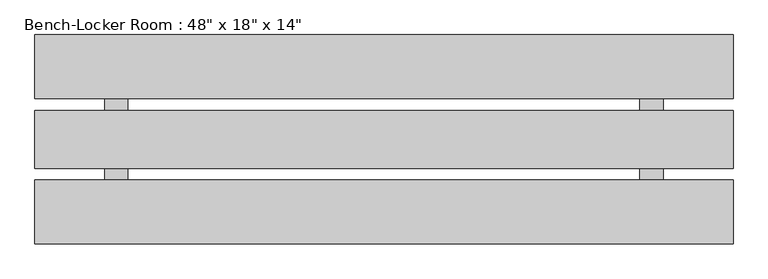
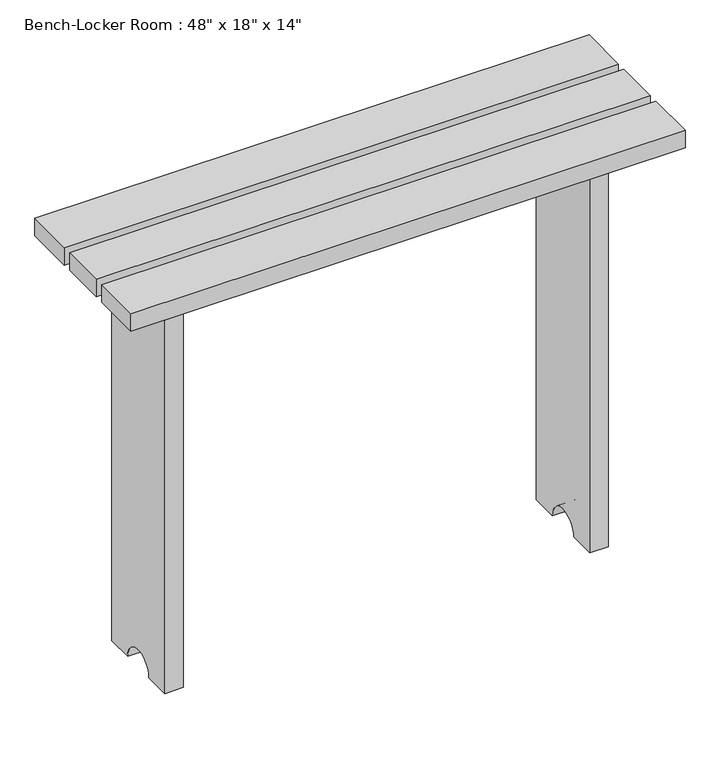
"""IFC4 building model written with IfcOpenShell, lengths in millimetres: furniture geometry."""

from ifc_helpers import new_model, si_unit, point, frame, frame_2d, origin, place, context, project, spatial, polyline, circle_curve, trimmed, segment, composite_curve, outline, extrude, source, transform, mapped, element, save


def furniture_f7008d8d(model_context):
    return source(origin(), model_context, "Body", "SweptSolid", [
        extrude(outline(polyline([(606.6852459, 47.8852459), (606.6852459, -91.8147541), (-917.3147541, -91.8147541), (-917.3147541, 47.8852459), (606.6852459, 47.8852459)])), frame((0.0, 0.0, 1168.4), z_axis=(0.0, 0.0, 1.0), x_axis=(1.0, 0.0, 0.0)), (0.0, 0.0, 1.0), 50.8),
        extrude(outline(polyline([(606.6852459, -409.3147541), (-917.3147541, -409.3147541), (-917.3147541, -269.6147541), (606.6852459, -269.6147541), (606.6852459, -409.3147541)])), frame((0.0, 0.0, 1168.4), z_axis=(0.0, 0.0, 1.0), x_axis=(1.0, 0.0, 0.0)), (0.0, 0.0, 1.0), 50.8),
        extrude(outline(polyline([(606.6852459, -117.2147541), (606.6852459, -244.2147541), (-917.3147541, -244.2147541), (-917.3147541, -117.2147541), (606.6852459, -117.2147541)])), frame((0.0, 0.0, 1168.4), z_axis=(0.0, 0.0, 1.0), x_axis=(1.0, 0.0, 0.0)), (0.0, 0.0, 1.0), 50.8),
        extrude(outline(composite_curve([segment(polyline([(-53.7147541, 0.0), (-129.9147541, 0.0)]), True, "CONTINUOUS"), segment(trimmed(circle_curve(frame_2d((-180.7147541, 0.0)), 50.8), [point((-129.9147541, 0.0))], [point((-231.5147541, 0.0))], True, "CARTESIAN"), True, "CONTINUOUS"), segment(polyline([(-231.5147541, 0.0), (-307.7147541, 0.0), (-307.7147541, 1168.4), (-53.7147541, 1168.4), (-53.7147541, 0.0)]), True, "CONTINUOUS")], self_intersect=False)), frame((-764.9147541, 0.0, 0.0), z_axis=(1.0, 0.0, 0.0), x_axis=(0.0, 1.0, 0.0)), (0.0, 0.0, 1.0), 50.8),
        extrude(outline(composite_curve([segment(polyline([(-307.7147541, 0.0), (-307.7147541, 1168.4), (-53.7147541, 1168.4), (-53.7147541, 0.0), (-129.9147541, 0.0)]), True, "CONTINUOUS"), segment(trimmed(circle_curve(frame_2d((-180.7147541, 0.0)), 50.8), [point((-129.9147541, 0.0))], [point((-231.5147541, 0.0))], True, "CARTESIAN"), True, "CONTINUOUS"), segment(polyline([(-231.5147541, 0.0), (-307.7147541, 0.0)]), True, "CONTINUOUS")], self_intersect=False)), frame((403.4852459, 0.0, 0.0), z_axis=(1.0, 0.0, 0.0), x_axis=(0.0, 1.0, 0.0)), (0.0, 0.0, 1.0), 50.8),
    ])


if __name__ == "__main__":
    model = new_model("IFC4")
    model_context = context("Model", 3, world=origin())
    ifc_project = project(units=[si_unit("LENGTHUNIT", "METRE", prefix="MILLI")], contexts=[model_context])
    site = spatial("IfcSite", under=ifc_project)
    building = spatial("IfcBuilding", under=site)
    placement = place(None, origin())
    furniture_shape = furniture_f7008d8d(model_context)
    element("IfcFurniture", 1, ObjectType="Bench-Locker Room : 48\" x 18\" x 14\"", at=placement, inside=building, context=model_context, shape_type="MappedRepresentation", body=[
        mapped(furniture_shape, transform((0.0, 0.0, 0.0), x_axis=(1.0, 0.0, 0.0), y_axis=(0.0, 1.0, 0.0), z_axis=(0.0, 0.0, 1.0))),
    ])
    save(model, "model.ifc")

# Revit data of these elements
# Type "Bench-Locker Room : 48\" x 18\" x 14\""
#   Assembly Code = "E2020200"
#   Depth = 1' - 6"
#   Height = 4' - 0"
#   Width = 5' - 0"
#   Bench Material = Cherry
#   Default Elevation = 0
# Element 1 (IfcFurniture, "Bench-Locker Room : 48\" x 18\" x 14\"")
#   Materials on its faces: "Cherry"
# Materials
#   "Cherry": class "Wood", colour RGB 226 177 128, transparency 0, Description = "Prunus Serotina", Cost = 0
